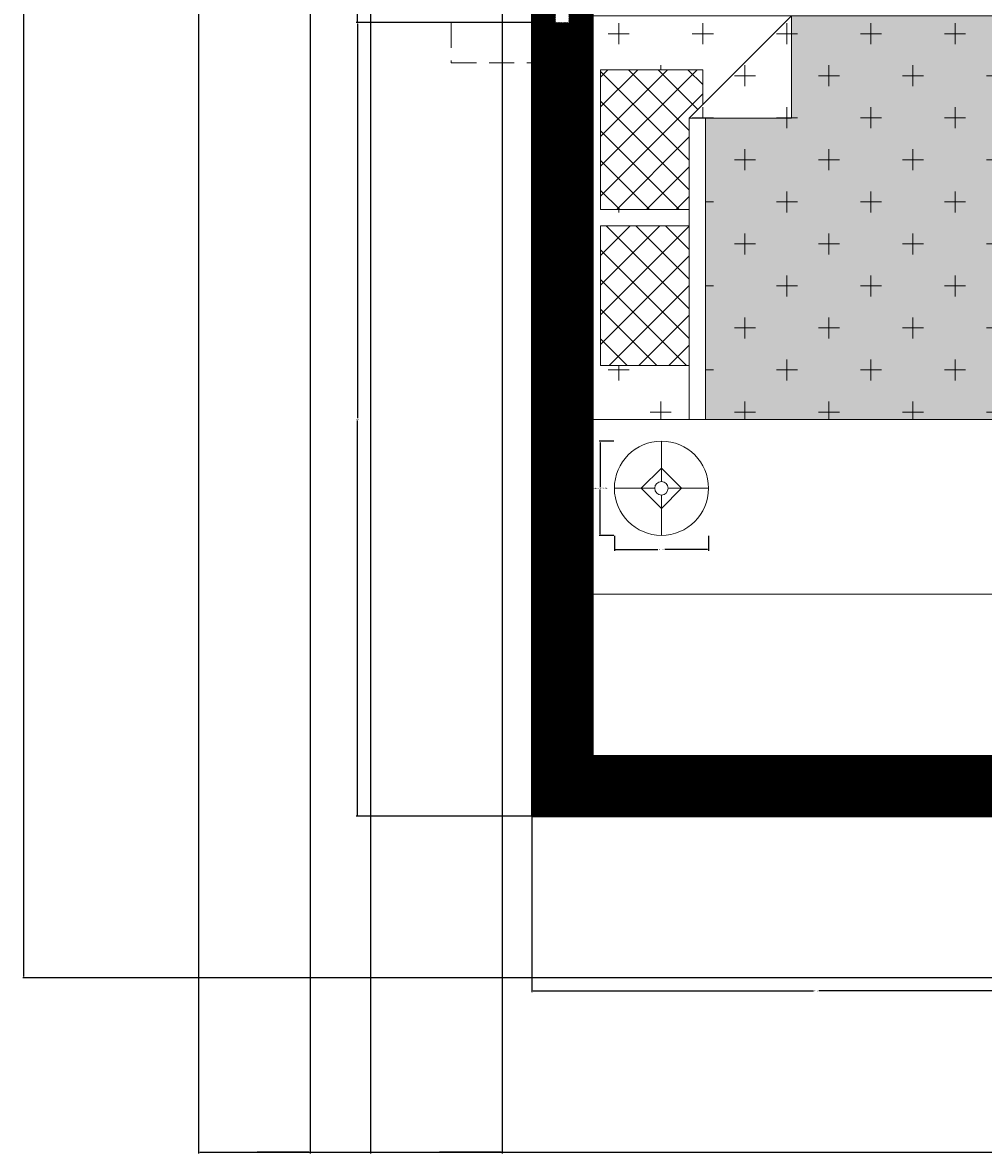
# Model space of a CAD drawing. Units: inches. Extents: x 557 to 1007, y 390 to 953.
# Tile 1 of 10: x 557 to 700, y 390 to 558. Entities that reach past the tile are written whole.
import ezdxf

# ---------------------------------------------------------------- set-up
doc = ezdxf.new("R2010")
doc.units = ezdxf.units.IN
doc.header["$LTSCALE"] = 5
doc.header["$MEASUREMENT"] = 0
doc.linetypes.add('HIDDEN', pattern=[0.375, 0.25, -0.125])
for name, color, linetype, lineweight in [('A-ANNO-DIMS', 2, 'Continuous', 18), ('A-FLOR-CASE', 8, 'Continuous', 18), ('A-FURN', 8, 'Continuous', 18), ('A-FURN-PATT', 9, 'Continuous', 9), ('A-GLAZ-OVHD', 8, 'HIDDEN', 13), ('A-WALL', 7, 'Continuous', 35), ('E-LITE', 2, 'Continuous', 13)]:
    doc.layers.add(name, color=color, linetype=linetype, lineweight=lineweight)
doc.layers.add('A-GLAZ-PATT', color=141, linetype='Continuous', lineweight=9, true_color=0xadddf7)
doc.layers.add('A-WALL-PATT', color=251, linetype='Continuous', lineweight=9, true_color=0x636466)
doc.styles.get("Standard").update_dxf_attribs({"font": 'arial.ttf'})
doc.dimstyles.get("Standard").update_dxf_attribs({"dimtxt": 0.18, "dimasz": 0.18, "dimexe": 0.18, "dimexo": 0.0625, "dimgap": 0.09, "dimtad": 0, "dimtih": 1, "dimtoh": 1, "dimdec": 4, "dimzin": 0, "dimdsep": 46, "dimtxsty": 'Standard', "dimcen": 0.09, "dimadec": 0, "dimazin": 0, "dimtfac": 1, "dimtdec": 4, "dimtofl": 0, "dimtmove": 0, "dimatfit": 3, "dimfxl": 1, "dimtolj": 1, "dimtzin": 0, "dimarcsym": 0})

# ---------------------------------------------------------------- blocks, each defined once
blk = doc.blocks.new('Lamp - Table')
for p, q in [((0, 7), (0, 1)), ((0, 3), (-3, 0)), ((3, 0), (0, 3)), ((-1, 0), (-7, 0)), ((-3, 0), (0, -3)), ((0, -3), (3, 0)), ((1, 0), (7, 0)), ((0, -1), (0, -7))]:
    blk.add_line(p, q)
for radius in [7, 1]:
    blk.add_circle((0, 0), radius)
blk = doc.blocks.new('BED-QUEEN-60x80-PLAN')
for p, q in [((0, 0), (0, 60)), ((0, 60), (80, 60)), ((29.6, 60), (14.4, 44.8)), ((29.6, 44.8), (29.6, 60)), ((80, 60), (80, 0)), ((1.2, 52), (16.4, 52)), ((1.2, 31.2), (1.2, 52)), ((16.4, 52), (16.4, 46.8)), ((14.4, 0), (14.4, 44.8)), ((14.4, 44.8), (29.6, 44.8)), ((16.8, 44.8), (16.8, 0)), ((14.4, 31.2), (1.2, 31.2)), ((1.2, 28.8), (14.4, 28.8)), ((1.2, 8), (1.2, 28.8)), ((14.4, 8), (1.2, 8)), ((80, 0), (0, 0))]:
    blk.add_line(p, q)
blk = doc.blocks.new('*D21')
at = {"layer": 'A-ANNO-DIMS', "color": 0, "lineweight": -2, "ltscale": 5, "transparency": 16777216}
for p, q in [((644.6, 495.67), (642.39, 495.67)), ((642.57, 495.49), (642.57, 488.85)), ((642.57, 481.85), (642.57, 488.49)), ((644.6, 481.67), (642.39, 481.67))]:
    blk.add_line(p, q, dxfattribs=at)
at = {"layer": 'A-ANNO-DIMS', "color": 0, "ltscale": 5, "transparency": 16777216}
for points in [[(642.54, 495.49), (642.6, 495.49), (642.57, 495.67)], [(642.54, 481.85), (642.6, 481.85), (642.57, 481.67)]]:
    blk.add_solid(points, dxfattribs=at)
at = {"layer": 'Defpoints', "color": 0, "ltscale": 5, "transparency": 16777216}
for p in [(642.57, 495.67), (644.67, 495.67), (644.67, 481.67)]:
    blk.add_point(p, dxfattribs=at)
at = {"layer": 'A-ANNO-DIMS', "color": 0, "ltscale": 5, "transparency": 16777216, "insert": (642.57, 488.67), "char_height": 0.18, "attachment_point": 5}
blk.add_mtext('\\A1;TABLE LAMP 14 TYP.', dxfattribs=at)
blk = doc.blocks.new('*D22')
at = {"layer": 'A-ANNO-DIMS', "color": 0, "lineweight": -2, "ltscale": 5, "transparency": 16777216}
for p, q in [((644.67, 481.6), (644.67, 479.39)), ((658.67, 481.6), (658.67, 479.39)), ((644.85, 479.57), (651.15, 479.57)), ((658.49, 479.57), (652.19, 479.57))]:
    blk.add_line(p, q, dxfattribs=at)
at = {"layer": 'A-ANNO-DIMS', "color": 0, "ltscale": 5, "transparency": 16777216}
for points in [[(644.85, 479.6), (644.85, 479.54), (644.67, 479.57)], [(658.49, 479.6), (658.49, 479.54), (658.67, 479.57)]]:
    blk.add_solid(points, dxfattribs=at)
at = {"layer": 'Defpoints', "color": 0, "ltscale": 5, "transparency": 16777216}
for p in [(644.67, 481.67), (658.67, 481.67), (644.67, 479.57)]:
    blk.add_point(p, dxfattribs=at)
at = {"layer": 'A-ANNO-DIMS', "color": 0, "ltscale": 5, "transparency": 16777216, "insert": (651.67, 479.57), "char_height": 0.18, "attachment_point": 5}
blk.add_mtext('\\A1;14 TYP.', dxfattribs=at)
blk = doc.blocks.new('*D45')
at = {"layer": 'A-ANNO-DIMS', "color": 0, "lineweight": -2, "ltscale": 5, "transparency": 16777216}
for p, q in [((582.82, 605.84), (582.82, 389.77)), ((980.41, 439.84), (980.41, 389.77)), ((583, 389.95), (781.22, 389.95)), ((980.23, 389.95), (782.01, 389.95))]:
    blk.add_line(p, q, dxfattribs=at)
at = {"layer": 'A-ANNO-DIMS', "color": 0, "ltscale": 5, "transparency": 16777216}
for points in [[(583, 389.98), (583, 389.92), (582.82, 389.95)], [(980.23, 389.98), (980.23, 389.92), (980.41, 389.95)]]:
    blk.add_solid(points, dxfattribs=at)
at = {"layer": 'Defpoints', "color": 0, "ltscale": 5, "transparency": 16777216}
for p in [(582.82, 605.9), (980.41, 439.9), (980.41, 389.95)]:
    blk.add_point(p, dxfattribs=at)
at = {"layer": 'A-ANNO-DIMS', "color": 0, "ltscale": 5, "transparency": 16777216, "insert": (781.61, 389.95), "char_height": 0.18, "attachment_point": 5}
blk.add_mtext('\\A1;397.6', dxfattribs=at)
blk = doc.blocks.new('*D46')
at = {"layer": 'A-ANNO-DIMS', "color": 0, "lineweight": -2, "ltscale": 5, "transparency": 16777216}
for p, q in [((761.34, 926.9), (556.69, 926.9)), ((556.87, 926.72), (556.87, 671.59)), ((556.87, 416.08), (556.87, 671.22)), ((773.34, 415.9), (556.69, 415.9))]:
    blk.add_line(p, q, dxfattribs=at)
at = {"layer": 'A-ANNO-DIMS', "color": 0, "ltscale": 5, "transparency": 16777216}
for points in [[(556.84, 926.72), (556.9, 926.72), (556.87, 926.9)], [(556.84, 416.08), (556.9, 416.08), (556.87, 415.9)]]:
    blk.add_solid(points, dxfattribs=at)
at = {"layer": 'Defpoints', "color": 0, "ltscale": 5, "transparency": 16777216}
for p in [(556.87, 926.9), (761.41, 926.9), (773.41, 415.9)]:
    blk.add_point(p, dxfattribs=at)
at = {"layer": 'A-ANNO-DIMS', "color": 0, "ltscale": 5, "transparency": 16777216, "insert": (556.87, 671.4), "char_height": 0.18, "attachment_point": 5}
blk.add_mtext('\\A1;511', dxfattribs=at)
blk = doc.blocks.new('*D64')
at = {"layer": 'A-ANNO-DIMS', "color": 0, "lineweight": -2, "ltscale": 5, "transparency": 16777216}
for p, q in [((632.34, 557.9), (606.28, 557.9)), ((606.46, 557.72), (606.46, 499.09)), ((606.46, 440.08), (606.46, 498.72)), ((632.34, 439.9), (606.28, 439.9))]:
    blk.add_line(p, q, dxfattribs=at)
at = {"layer": 'A-ANNO-DIMS', "color": 0, "ltscale": 5, "transparency": 16777216}
for points in [[(606.43, 557.72), (606.49, 557.72), (606.46, 557.9)], [(606.43, 440.08), (606.49, 440.08), (606.46, 439.9)]]:
    blk.add_solid(points, dxfattribs=at)
at = {"layer": 'Defpoints', "color": 0, "ltscale": 5, "transparency": 16777216}
for p in [(606.46, 557.9), (632.41, 557.9), (632.41, 439.9)]:
    blk.add_point(p, dxfattribs=at)
at = {"layer": 'A-ANNO-DIMS', "color": 0, "ltscale": 5, "transparency": 16777216, "insert": (606.46, 498.9), "char_height": 0.18, "attachment_point": 5}
blk.add_mtext('\\A1;118', dxfattribs=at)
blk = doc.blocks.new('*D65')
at = {"layer": 'A-ANNO-DIMS', "color": 0, "lineweight": -2, "ltscale": 5, "transparency": 16777216}
for p, q in [((632.34, 593.9), (606.28, 593.9)), ((606.46, 593.72), (606.46, 576.09)), ((606.46, 558.08), (606.46, 575.72)), ((632.34, 557.9), (606.28, 557.9))]:
    blk.add_line(p, q, dxfattribs=at)
at = {"layer": 'A-ANNO-DIMS', "color": 0, "ltscale": 5, "transparency": 16777216}
for points in [[(606.43, 593.72), (606.49, 593.72), (606.46, 593.9)], [(606.43, 558.08), (606.49, 558.08), (606.46, 557.9)]]:
    blk.add_solid(points, dxfattribs=at)
at = {"layer": 'Defpoints', "color": 0, "ltscale": 5, "transparency": 16777216}
for p in [(606.46, 593.9), (632.41, 593.9), (632.41, 557.9)]:
    blk.add_point(p, dxfattribs=at)
at = {"layer": 'A-ANNO-DIMS', "color": 0, "ltscale": 5, "transparency": 16777216, "insert": (606.46, 575.9), "char_height": 0.18, "attachment_point": 5}
blk.add_mtext('\\A1;36', dxfattribs=at)
blk = doc.blocks.new('*D68')
at = {"layer": 'A-ANNO-DIMS', "color": 0, "lineweight": -2, "ltscale": 5, "transparency": 16777216}
for p, q in [((632.41, 439.84), (632.41, 413.77)), ((716.96, 439.84), (716.96, 413.77)), ((632.59, 413.95), (674.29, 413.95)), ((716.78, 413.95), (675.08, 413.95))]:
    blk.add_line(p, q, dxfattribs=at)
at = {"layer": 'A-ANNO-DIMS', "color": 0, "ltscale": 5, "transparency": 16777216}
for points in [[(632.59, 413.98), (632.59, 413.92), (632.41, 413.95)], [(716.78, 413.98), (716.78, 413.92), (716.96, 413.95)]]:
    blk.add_solid(points, dxfattribs=at)
at = {"layer": 'Defpoints', "color": 0, "ltscale": 5, "transparency": 16777216}
for p in [(632.41, 439.9), (716.96, 439.9), (632.41, 413.95)]:
    blk.add_point(p, dxfattribs=at)
at = {"layer": 'A-ANNO-DIMS', "color": 0, "ltscale": 5, "transparency": 16777216, "insert": (674.68, 413.95), "char_height": 0.18, "attachment_point": 5}
blk.add_mtext('\\A1;84.55', dxfattribs=at)
blk = doc.blocks.new('*D75')
at = {"layer": 'A-ANNO-DIMS', "color": 0, "lineweight": -2, "ltscale": 5, "transparency": 16777216}
for p, q in [((582.82, 614.84), (582.82, 389.77)), ((599.41, 614.84), (599.41, 389.77)), ((583, 389.95), (590.66, 389.95)), ((599.23, 389.95), (591.57, 389.95))]:
    blk.add_line(p, q, dxfattribs=at)
at = {"layer": 'A-ANNO-DIMS', "color": 0, "ltscale": 5, "transparency": 16777216}
for points in [[(583, 389.98), (583, 389.92), (582.82, 389.95)], [(599.23, 389.98), (599.23, 389.92), (599.41, 389.95)]]:
    blk.add_solid(points, dxfattribs=at)
at = {"layer": 'Defpoints', "color": 0, "ltscale": 5, "transparency": 16777216}
for p in [(582.82, 614.9), (599.41, 614.9), (582.82, 389.95)]:
    blk.add_point(p, dxfattribs=at)
at = {"layer": 'A-ANNO-DIMS', "color": 0, "ltscale": 5, "transparency": 16777216, "insert": (591.11, 389.95), "char_height": 0.18, "attachment_point": 5}
blk.add_mtext('\\A1;16.582', dxfattribs=at)
blk = doc.blocks.new('*D91')
at = {"layer": 'A-ANNO-DIMS', "color": 0, "lineweight": -2, "ltscale": 5, "transparency": 16777216}
for p, q in [((628, 688.44), (628, 389.77)), ((608.41, 614.84), (608.41, 389.77)), ((608.59, 389.95), (617.75, 389.95)), ((627.82, 389.95), (618.66, 389.95))]:
    blk.add_line(p, q, dxfattribs=at)
at = {"layer": 'A-ANNO-DIMS', "color": 0, "ltscale": 5, "transparency": 16777216}
for points in [[(608.59, 389.98), (608.59, 389.92), (608.41, 389.95)], [(627.82, 389.98), (627.82, 389.92), (628, 389.95)]]:
    blk.add_solid(points, dxfattribs=at)
at = {"layer": 'Defpoints', "color": 0, "ltscale": 5, "transparency": 16777216}
for p in [(628, 688.5), (608.41, 614.9), (608.41, 389.95)]:
    blk.add_point(p, dxfattribs=at)
at = {"layer": 'A-ANNO-DIMS', "color": 0, "ltscale": 5, "transparency": 16777216, "insert": (618.2, 389.95), "char_height": 0.18, "attachment_point": 5}
blk.add_mtext('\\A1;19.595', dxfattribs=at)

msp = doc.modelspace()

# ---------------------------------------------------------------- hatches: boundary and pattern name
at = {"layer": 'A-FURN-PATT', "ltscale": 5}
h = msp.add_hatch(dxfattribs=at)
h.set_pattern_fill('GRAVEL', color=256, scale=25)
h.set_pattern_definition([(228.01279, (18, 25), (-200, -225), [3.3634, -332.9772]), (184.96974, (15.75, 22.5), (300, 25), [5.7717, -571.39812]), (132.51045, (10, 22), (250, -275), [4.0697, -402.9008]), (267.27369, (0.25, 15.75), (25, 500), [5.25595, -520.33895]), (292.83365, (0, 10.5), (-125, 300), [5.15387, -510.23433]), (357.27369, (2, 5.75), (-500, 25), [5.25595, -520.33895]), (37.69424, (7.25, 5.5), (-325, -250), [6.95072, -688.1212]), (72.25533, (12.75, 9.75), (175, 550), [6.5622, -649.65804]), (121.42957, (14.75, 16), (-200, 325), [5.27375, -522.10183]), (175.23636, (12, 20.5), (275, -25), [6.0208, -295.01906]), (222.39744, (6, 21), (-300, -275), [7.7862, -770.83438]), (138.81407, (25, 15.5), (-175, 150), [2.65752, -263.0961]), (171.46923, (23, 17.25), (325, -50), [5.05593, -500.5378]), (225, (18, 18), (-3e-15, -25), [3.53552, -31.8198]), (203.1986, (16.25, 21), (125, 50), [1.90395, -188.49038]), (291.8014, (14.5, 20.25), (-25, 75), [2.69257, -131.93655]), (30.96376, (15.5, 17.75), (75, 50), [4.37322, -141.40057]), (161.56505, (19.25, 20), (50, -25), [3.16228, -75.89467]), (16.38954, (0, 20.25), (250, 75), [4.43, -438.57113]), (70.34618, (4.25, 21.5), (-100, -275), [3.71652, -367.9352]), (293.1986, (19.25, 25), (-50, 125), [3.80788, -186.58645]), (343.61046, (20.75, 21.5), (-250, 75), [4.43, -438.57113]), (339.44395, (0, 4.75), (-125, 50), [4.272, -209.3281]), (294.77514, (4, 3.25), (-125, 275), [3.57945, -354.36608]), (66.8014, (19.5, 0), (50, 125), [3.80788, -186.58645]), (17.35402, (21, 3.5), (-325, -100), [4.19078, -414.8856]), (69.44395, (7.25, 0), (-50, -125), [2.136, -211.4641]), (101.30993, (18, 0), (-25, 100), [1.27475, -126.20074]), (165.96376, (17.75, 1.25), (75, -25), [5.15388, -97.92377]), (186.00901, (12.75, 2.5), (250, 25), [4.77625, -472.84808]), (303.69007, (15.5, 15.5), (-25, 50), [3.60555, -86.53323]), (353.15723, (17.5, 12.5), (425, -50), [6.29485, -623.18907]), (60.9454, (23.75, 11.75), (-100, -175), [2.5739, -254.81685]), (90, (25, 14), (-25, 25), [1.5, -23.5]), (120.25644, (12.25, 3.25), (100, -175), [3.4731, -343.838]), (48.01279, (10.5, 6.25), (200, 225), [6.7268, -329.6138]), (0, (15, 11.25), (25, 25), [6.5, -18.5]), (325.30485, (21.5, 11.25), (250, -175), [3.95285, -391.33186]), (254.0546, (24.75, 9), (-25, -100), [3.64005, -178.3627]), (207.64598, (23.75, 5.5), (-475, -250), [5.92662, -586.73685]), (175.42608, (18.5, 2.75), (-325, 25), [6.26997, -620.72684])])
h.paths.add_polyline_path([(615.2525, 688.5, 1), (640.7475, 688.5, 1)])
h.paths.add_polyline_path([(917.0544, 663.8414, 0.33333323), (915.2241, 665.6717), (882.2793, 665.6717, 0.33333323), (880.449, 663.8414), (880.449, 649.1992, 0.33333323), (882.2793, 647.369), (915.2241, 647.369, 0.33333323), (917.0544, 649.1992)])
h.paths.add_polyline_path([(828.0807, 699.7098), (756.0807, 699.7098), (756.0807, 663.7098), (828.0807, 663.7098)])
h.paths.add_polyline_path([(787.5651, 663.7098), (768.5964, 663.7098), (769.8463, 655.7098), (786.3151, 655.7098)])
h.paths.add_polyline_path([(815.5651, 663.7098), (796.5964, 663.7098), (797.8463, 655.7098), (814.3151, 655.7098)])
h.paths.add_polyline_path([(836.0807, 689.9442), (828.0807, 691.1942), (828.0807, 672.2255), (836.0807, 673.4755)])
h.paths.add_polyline_path([(756.0807, 691.1942), (748.0807, 689.9442), (748.0807, 673.4755), (756.0807, 672.2255)])
h.paths.add_polyline_path([(786.3151, 707.7098), (769.8463, 707.7098), (768.5964, 699.7098), (787.5651, 699.7098)])
h.paths.add_polyline_path([(814.3151, 707.7098), (797.8463, 707.7098), (796.5964, 699.7098), (815.5651, 699.7098)])
h.paths.add_polyline_path([(917.4362, 607.3575), (889.5896, 607.3575), (889.5896, 586.4726), (917.4362, 586.4726)])
h.paths.add_polyline_path([(721.4053, 881.8539), (671.0053, 881.8539), (671.0053, 866.6539), (658.2053, 866.6539), (658.2053, 821.8539), (721.4053, 821.8539)])
h.paths.add_polyline_path([(925.4053, 875.1046), (875.0053, 875.1046), (875.0053, 859.9046), (862.2053, 859.9046), (862.2053, 815.1046), (925.4053, 815.1046)])
h.paths.add_polyline_path([(721.4053, 558.9046), (671.0053, 558.9046), (671.0053, 543.7046), (658.2053, 543.7046), (658.2053, 498.9046), (721.4053, 498.9046)])
at = {"layer": 'A-FURN-PATT'}
h = msp.add_hatch(dxfattribs=at)
h.set_pattern_fill('CROSS', color=256, scale=25)
h.paths.add_polyline_path([(925.4053, 875.1046), (875.0053, 875.1046), (875.0053, 859.9046), (862.2053, 859.9046), (862.2053, 815.1046), (925.4053, 815.1046)])
h.paths.add_polyline_path([(721.4053, 881.8539), (671.0053, 881.8539), (671.0053, 866.6539), (658.2053, 866.6539), (658.2053, 821.8539), (721.4053, 821.8539)])
h.paths.add_polyline_path([(671.0053, 881.8539), (655.8053, 866.6539), (671.0053, 866.6539)], flags=17)
h.paths.add_polyline_path([(671.0053, 881.8539), (641.4053, 881.8539), (641.4053, 821.8539), (655.8053, 821.8539), (655.8053, 829.8539), (642.6053, 829.8539), (642.6053, 850.6539), (655.8053, 850.6539), (655.8053, 853.0539), (642.6053, 853.0539), (642.6053, 873.8539), (657.8053, 873.8539), (657.8053, 868.6539)])
h.paths.add_polyline_path([(875.0053, 875.1046), (859.8053, 859.9046), (875.0053, 859.9046)], flags=17)
h.paths.add_polyline_path([(875.0053, 875.1046), (845.4053, 875.1046), (845.4053, 815.1046), (859.8053, 815.1046), (859.8053, 823.1046), (846.6053, 823.1046), (846.6053, 843.9046), (859.8053, 843.9046), (859.8053, 846.3046), (846.6053, 846.3046), (846.6053, 867.1046), (861.8053, 867.1046), (861.8053, 861.9046)])
h.paths.add_polyline_path([(721.4053, 558.9046), (671.0053, 558.9046), (671.0053, 543.7046), (658.2053, 543.7046), (658.2053, 498.9046), (721.4053, 498.9046)])
h.paths.add_polyline_path([(671.0053, 558.9046), (641.4053, 558.9046), (641.4053, 498.9046), (655.8053, 498.9046), (655.8053, 506.9046), (642.6053, 506.9046), (642.6053, 527.7046), (655.8053, 527.7046), (655.8053, 530.1046), (642.6053, 530.1046), (642.6053, 550.9046), (657.8053, 550.9046), (657.8053, 545.7046)])
h.paths.add_polyline_path([(671.0053, 558.9046), (657.8053, 545.7046), (655.8053, 543.7046), (671.0053, 543.7046)], flags=17)
h.paths.add_polyline_path([(873.1461, 661.8773, 0.41421356), (868.1461, 666.8773, -0.12244426), (867.1516, 666.8773), (855.014, 666.8773), (855.014, 647.2429), (867.4581, 647.2429, -0.08537395), (868.1461, 647.2429, 0.41421356), (873.1461, 652.2429)])
h.paths.add_polyline_path([(917.0544, 663.8414, 0.33333323), (915.2241, 665.6717), (882.2793, 665.6717, 0.33333323), (880.449, 663.8414), (880.449, 649.1992, 0.33333323), (882.2793, 647.369), (915.2241, 647.369, 0.33333323), (917.0544, 649.1992)])
h.paths.add_polyline_path([(944.9465, 667.5202), (932.6561, 667.5202, -0.10407786), (931.8144, 667.5202, 0.41421356), (926.8144, 662.5202), (926.8144, 652.8858, 0.41421356), (931.8144, 647.8858, -0.05611627), (932.2647, 647.8858), (944.9465, 647.8858)])
h.paths.add_polyline_path([(928.8341, 635.542, 0.41421356), (923.8341, 640.542), (914.1997, 640.542, 0.41421356), (909.1997, 635.542), (909.1997, 622.4099), (923.8341, 622.4099, 0.41421356), (928.8341, 627.4099)])
h.paths.add_polyline_path([(909.1997, 635.542, 0.41421356), (904.1997, 640.542), (894.5653, 640.542, 0.41421356), (889.5653, 635.542), (889.5653, 622.4099), (909.1997, 622.4099)])
h.paths.add_polyline_path([(889.5653, 635.542, 0.41421356), (884.5653, 640.542), (874.9308, 640.542, 0.41421356), (869.9308, 635.542), (869.9308, 627.4099, 0.41421356), (874.9308, 622.4099), (889.5653, 622.4099)])
h = msp.add_hatch(dxfattribs=at)
h.set_pattern_fill('ANSI37', color=256, scale=25)
h.paths.add_polyline_path([(655.8053, 866.6539), (657.8053, 868.6539), (657.8053, 873.8539), (642.6053, 873.8539), (642.6053, 853.0539), (655.8053, 853.0539)])
h.paths.add_polyline_path([(655.8053, 850.6539), (642.6053, 850.6539), (642.6053, 829.8539), (655.8053, 829.8539)])
h.paths.add_polyline_path([(859.8053, 859.9046), (861.8053, 861.9046), (861.8053, 867.1046), (846.6053, 867.1046), (846.6053, 846.3046), (859.8053, 846.3046)])
h.paths.add_polyline_path([(859.8053, 843.9046), (846.6053, 843.9046), (846.6053, 823.1046), (859.8053, 823.1046)])
h.paths.add_polyline_path([(655.8053, 527.7046), (642.6053, 527.7046), (642.6053, 506.9046), (655.8053, 506.9046)])
h.paths.add_polyline_path([(657.8053, 545.7046), (657.8053, 550.9046), (642.6053, 550.9046), (642.6053, 530.1046), (655.8053, 530.1046), (655.8053, 543.7046)])
at = {"layer": 'A-GLAZ-PATT'}
h = msp.add_hatch(dxfattribs=at)
h.set_pattern_fill('ANSI31', color=256)
h.paths.add_polyline_path([(635.9053, 814.7688), (636.9053, 814.7688), (636.9053, 838.7688), (632.4053, 838.7688), (632.4053, 790.7688), (635.9053, 790.7688)])
h.paths.add_polyline_path([(641.4053, 838.7688), (637.9053, 838.7688), (637.9053, 814.7688), (636.9053, 814.7688), (636.9053, 790.7688), (641.4053, 790.7688)])
h.paths.add_polyline_path([(603.4053, 728.9046, -0.41421356), (623.4053, 748.9046), (632.4053, 748.9046), (632.4053, 752.9046), (623.4053, 752.9046, 0.41421356), (599.4053, 728.9046), (599.4053, 614.9046), (603.4053, 614.9046)])
h.paths.add_polyline_path([(632.4053, 743.9046), (632.4053, 747.9046), (623.4053, 747.9046, 0.41421356), (604.4053, 728.9046), (604.4053, 614.9046), (608.4053, 614.9046), (608.4053, 719.9046, -0.41421356)])
h.paths.add_polyline_path([(683.4053, 722.9046), (678.9053, 722.9046), (678.9053, 698.9046), (679.9053, 698.9046), (679.9053, 662.9046), (678.9053, 662.9046), (678.9053, 638.9046), (683.4053, 638.9046)])
h.paths.add_polyline_path([(678.9053, 698.9046), (677.9053, 698.9046), (677.9053, 722.9046), (674.4053, 722.9046), (674.4053, 638.9046), (677.9053, 638.9046), (677.9053, 662.9046), (678.9053, 662.9046)])
h.paths.add_polyline_path([(635.9053, 593.9046), (632.4053, 593.9046), (632.4053, 557.9046), (635.9053, 557.9046)])
h.paths.add_polyline_path([(641.4053, 593.9046), (637.9053, 593.9046), (637.9053, 557.9046), (641.4053, 557.9046)])
h.paths.add_polyline_path([(764.9579, 448.9046), (716.9579, 448.9046), (716.9579, 445.4046), (740.9579, 445.4046), (740.9579, 444.4046), (764.9579, 444.4046)])
h.paths.add_polyline_path([(764.9579, 443.4046), (740.9579, 443.4046), (740.9579, 444.4046), (716.9579, 444.4046), (716.9579, 439.9046), (764.9579, 439.9046)])
h.paths.add_polyline_path([(938.4053, 905.9046), (878.4053, 905.9046), (878.4053, 902.4046), (908.4053, 902.4046), (908.4053, 901.4046), (938.4053, 901.4046)])
h.paths.add_polyline_path([(938.4053, 900.4046), (908.4053, 900.4046), (908.4053, 901.4046), (878.4053, 901.4046), (878.4053, 896.9046), (938.4053, 896.9046)])
h.paths.add_polyline_path([(724.9087, 905.9046), (676.9087, 905.9046), (676.9087, 902.4046), (701.4053, 902.4046), (701.4053, 901.4046), (724.9087, 901.4046)])
h.paths.add_polyline_path([(724.9087, 900.4046), (701.4053, 900.4046), (701.4053, 901.4046), (676.9087, 901.4046), (676.9087, 896.9046), (724.9087, 896.9046)])
h.paths.add_polyline_path([(832.0625, 905.9046), (808.0625, 905.9046), (808.0625, 902.4046), (832.0625, 902.4046)])
h.paths.add_polyline_path([(832.0625, 900.4046), (808.0625, 900.4046), (808.0625, 896.9046), (832.0625, 896.9046)])
at = {"layer": 'A-WALL-PATT'}
h = msp.add_hatch(dxfattribs=at)
h.set_pattern_fill('ANSI31', color=256)
h.paths.add_polyline_path([(808.0625, 905.9046), (767.4053, 905.9046), (767.4053, 920.9046), (839.4053, 920.9046), (839.4053, 905.9046), (832.0625, 905.9046), (832.0625, 896.9046), (839.4053, 896.9046), (839.4053, 800.9046), (837.4053, 800.9046), (837.4053, 794.9046), (839.4053, 794.9046), (839.4053, 790.9046), (845.4053, 790.9046), (845.4053, 896.9046), (878.4053, 896.9046), (878.4053, 905.9046), (845.4053, 905.9046), (845.4053, 926.9046), (761.4053, 926.9046), (761.4053, 914.9046), (761.4053, 905.9046), (724.9087, 905.9046), (724.9087, 896.9046), (761.4053, 896.9046), (761.4053, 752.9046), (759.4053, 752.9046), (759.4053, 746.9046), (767.4053, 746.9046), (767.4053, 794.9046), (807.4053, 794.9046), (807.4053, 800.9046), (767.4053, 800.9046), (767.4053, 896.9046), (808.0625, 896.9046)])
h.paths.add_polyline_path([(676.9087, 905.9046), (632.4053, 905.9046), (632.4053, 838.7688), (641.4053, 838.7688), (641.4053, 881.8539), (641.4053, 896.9046), (676.9087, 896.9046)])
h.paths.add_polyline_path([(980.4053, 905.9046), (938.4053, 905.9046), (938.4053, 896.9046), (971.4053, 896.9046), (971.4053, 752.9046), (845.4053, 752.9046), (845.4053, 754.9046), (839.4053, 754.9046), (839.4053, 746.9046), (971.4053, 746.9046), (971.4053, 720.1788), (980.4053, 720.1788)])
h.paths.add_polyline_path([(723.4053, 752.9046), (641.4053, 752.9046), (641.4053, 790.7688), (632.4053, 790.7688), (632.4053, 743.9046), (674.4053, 743.9046), (674.4053, 722.9046), (683.4053, 722.9046), (683.4053, 746.9046), (723.4053, 746.9046)])
h.paths.add_polyline_path([(980.4053, 684.1788), (971.4053, 684.1788), (971.4053, 614.9046), (845.4053, 614.9046), (845.4053, 608.9046), (971.4053, 608.9046), (971.4053, 512.9046), (908.7697, 512.9046), (908.7697, 508.9046), (971.4053, 508.9046), (971.4053, 448.9046), (845.4053, 448.9046), (845.4053, 508.9046), (878.7697, 508.9046), (878.7697, 512.9046), (845.4053, 512.9046), (845.4053, 562.9046), (779.4053, 562.9046), (779.4053, 614.9046), (761.4053, 614.9046), (761.4053, 608.9046), (773.4053, 608.9046), (773.4053, 512.636), (779.4053, 512.636), (779.4053, 556.9046), (839.4053, 556.9046), (839.4053, 448.9046), (830.432, 448.9046), (830.432, 439.9046), (839.4053, 439.9046), (839.4053, 433.0506), (839.4053, 421.9046), (779.4053, 421.9046), (779.4053, 439.9046), (796.9656, 439.9046), (806.432, 439.9046), (806.432, 448.9046), (779.4053, 448.9046), (779.4053, 482.636), (773.4053, 482.636), (773.4053, 448.9046), (764.9579, 448.9046), (764.9579, 439.9046), (773.4053, 439.9046), (773.4053, 415.9046), (845.4053, 415.9046), (845.4053, 439.9046), (980.4053, 439.9046)])
h.paths.add_polyline_path([(716.9579, 448.9046), (641.4053, 448.9046), (641.4053, 557.9046), (632.4053, 557.9046), (632.4053, 439.9046), (716.9579, 439.9046)])
h.paths.add_polyline_path([(725.4053, 614.9046), (683.4053, 614.9046), (683.4053, 638.9046), (674.4053, 638.9046), (674.4053, 614.9046), (608.4053, 614.9046), (582.8236, 614.9046), (582.8236, 605.9046), (599.4053, 605.9046), (632.4053, 605.9046), (641.4053, 605.9046), (641.4053, 608.9046), (725.4053, 608.9046)])
h.paths.add_polyline_path([(641.4053, 605.9046), (632.4053, 605.9046), (632.4053, 593.9046), (641.4053, 593.9046)])

# ---------------------------------------------------------------- linework, layer by layer
at = {"layer": 'A-FLOR-CASE'}
msp.add_line((641.4053, 472.9046), (773.4053, 472.9046), dxfattribs=at)
at = {"layer": 'A-GLAZ-OVHD', "ltscale": 3}
for p, q in [((620.4053, 557.9046), (620.4053, 551.9046)), ((620.4053, 551.9046), (632.4053, 551.9046))]:
    msp.add_line(p, q, dxfattribs=at)
at = {"layer": 'A-WALL'}
for p, q in [((641.4053, 608.9046), (641.4053, 448.9046)), ((632.4053, 605.9046), (632.4053, 439.9046)), ((641.4053, 448.9046), (773.4053, 448.9046)), ((632.4053, 439.9046), (773.4053, 439.9046))]:
    msp.add_line(p, q, dxfattribs=at)

# ---------------------------------------------------------------- block references
at = {"layer": 'A-FURN'}
msp.add_blockref('BED-QUEEN-60x80-PLAN', (641.405, 498.905), dxfattribs=at)
at = {"layer": 'E-LITE', "rotation": 90}
msp.add_blockref('Lamp - Table', (651.666, 488.6659), dxfattribs=at)

# ---------------------------------------------------------------- dimensions: what is measured, and where the dimension line sits
at = {"layer": 'A-ANNO-DIMS', "ltscale": 5}
for base, p1, p2, angle, override, picture, middle in [((556.8736, 926.9046), (773.4053, 415.9046), (761.4053, 926.9046), 90, {"dimdec": 0, "dimlfac": 1, "dimrnd": 0, "dimzin": 0, "dimdsep": 46, "dimlunit": 2}, '*D46', (556.8736, 671.4046)), ((606.4553, 593.9046), (632.4053, 557.9046), (632.4053, 593.9046), 90, {"dimdec": 0, "dimlfac": 1, "dimrnd": 0, "dimzin": 0, "dimdsep": 46, "dimlunit": 2}, '*D65', (606.4553, 575.9046)), ((606.4553, 557.9046), (632.4053, 439.9046), (632.4053, 557.9046), 90, {"dimdec": 0, "dimlfac": 1, "dimrnd": 0, "dimzin": 0, "dimdsep": 46, "dimlunit": 2}, '*D64', (606.4553, 498.9046)), ((632.4053, 413.9546), (716.9579, 439.9046), (632.4053, 439.9046), 180, {"dimdec": 2, "dimlfac": 1, "dimrnd": 0, "dimzin": 0, "dimdsep": 46, "dimlunit": 2}, '*D68', (674.6816, 413.9546))]:
    dim = msp.add_linear_dim(base=base, p1=p1, p2=p2, angle=angle, dimstyle='Standard', override=override, dxfattribs=at)
    dim.commit()
    dim.dimension.update_dxf_attribs({"geometry": picture, "text_midpoint": middle})
for base, p1, p2, override, picture, middle in [((608.4053, 389.9546), (628, 688.5), (608.4053, 614.9046), {"dimdec": 3, "dimlfac": 1, "dimrnd": 0, "dimzin": 0, "dimdsep": 46, "dimlunit": 2}, '*D91', (618.2026, 389.9546)), ((582.8236, 389.9546), (599.4053, 614.9046), (582.8236, 614.9046), {"dimdec": 3, "dimlfac": 1, "dimrnd": 0, "dimzin": 0, "dimdsep": 46, "dimlunit": 2}, '*D75', (591.1144, 389.9546)), ((980.4053, 389.9546), (582.8236, 605.9046), (980.4053, 439.9046), {"dimdec": 1, "dimlfac": 1, "dimrnd": 0, "dimzin": 0, "dimdsep": 46, "dimlunit": 2}, '*D45', (781.6144, 389.9546))]:
    dim = msp.add_linear_dim(base=base, p1=p1, p2=p2, dimstyle='Standard', override=override, dxfattribs=at)
    dim.commit()
    dim.dimension.update_dxf_attribs({"geometry": picture, "text_midpoint": middle})
for base, p1, p2, angle, text, picture, middle in [((642.566, 495.6659), (644.666, 481.6659), (644.666, 495.6659), 90, 'TABLE LAMP <> TYP.', '*D21', (642.566, 488.6659)), ((644.666, 479.5659), (658.666, 481.6659), (644.666, 481.6659), 180, '<> TYP.', '*D22', (651.666, 479.5659))]:
    dim = msp.add_linear_dim(base=base, p1=p1, p2=p2, angle=angle, text=text, dimstyle='Standard', override={"dimdec": 0, "dimlfac": 1, "dimrnd": 0, "dimzin": 0, "dimdsep": 46, "dimlunit": 2}, dxfattribs=at)
    dim.commit()
    dim.dimension.update_dxf_attribs({"geometry": picture, "text_midpoint": middle})

doc.saveas('drawing.dxf')
